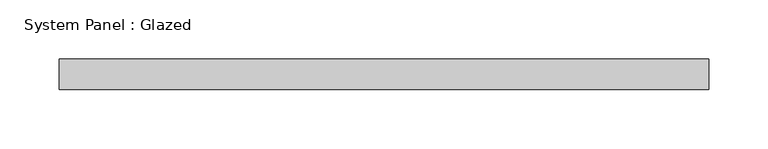
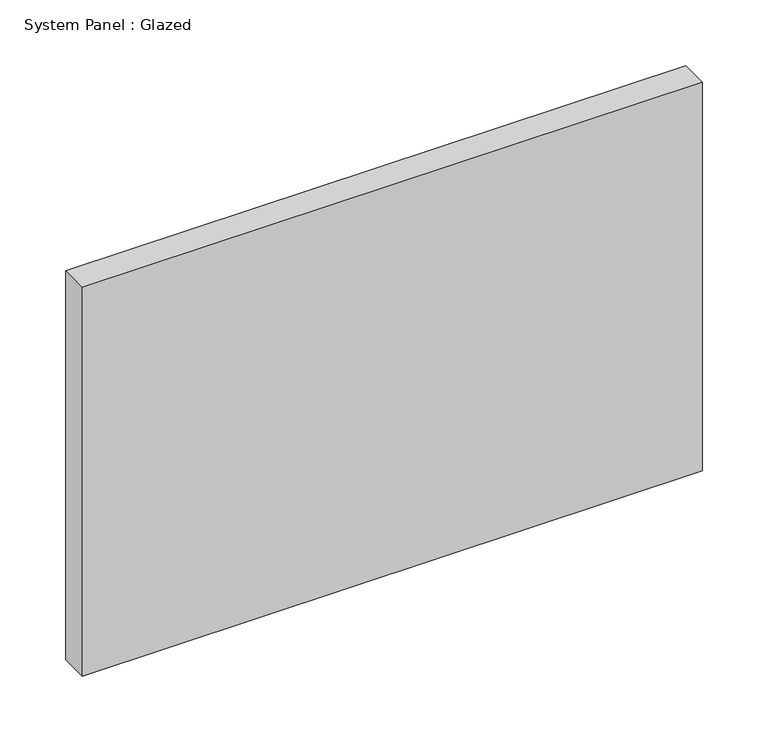
"""IFC4 building model written with IfcOpenShell, lengths in millimetres: plate geometry, System Panel : Glazed."""

from ifc_helpers import new_model, si_unit, origin, origin_with_axes, place, context, project, spatial, polyline, outline, extrude, source, transform, mapped, element, save


def system_panel_glazed_398ce57b(model_context):
    return source(origin(), model_context, "Body", "SweptSolid", [
        extrude(outline(polyline([(273.05, 19.05), (-273.05, 19.05), (-273.05, 44.45), (273.05, 44.45), (273.05, 19.05)])), origin_with_axes(), (0.0, 0.0, 1.0), 361.95),
    ])


if __name__ == "__main__":
    model = new_model("IFC4")
    model_context = context("Model", 3, world=origin())
    ifc_project = project(units=[si_unit("LENGTHUNIT", "METRE", prefix="MILLI")], contexts=[model_context])
    site = spatial("IfcSite", under=ifc_project)
    building = spatial("IfcBuilding", under=site)
    placement = place(None, origin())
    system_panel_glazed_shape = system_panel_glazed_398ce57b(model_context)
    element("IfcPlate", 1, ObjectType="System Panel : Glazed", at=placement, inside=building, context=model_context, shape_type="MappedRepresentation", body=[
        mapped(system_panel_glazed_shape, transform((0.0, 0.0, 0.0), x_axis=(1.0, 0.0, 0.0), y_axis=(0.0, 1.0, 0.0), z_axis=(0.0, 0.0, 1.0))),
    ])
    save(model, "model.ifc")

# Revit data of these elements
# Type "System Panel : Glazed"
#   Construction Type Id = "GSP4R"
#   Analytic Construction = "1/8 in Pilkington single glazing"
#   Visual Light Transmittance = 0.9
#   Solar Heat Gain Coefficient = 0.86
#   Heat Transfer Coefficient (U) = 1.18115 BTU/(h·ft²·°F)
#   Define Thermal Properties by = 1
# Element 1 (IfcPlate, "System Panel : Glazed")
#   Materials on its faces: "Glass"
# Materials
#   "Glass": class "Glass", colour RGB 0 128 192, transparency 0.75, Description = "Soda Lime Glass", Cost = 0
